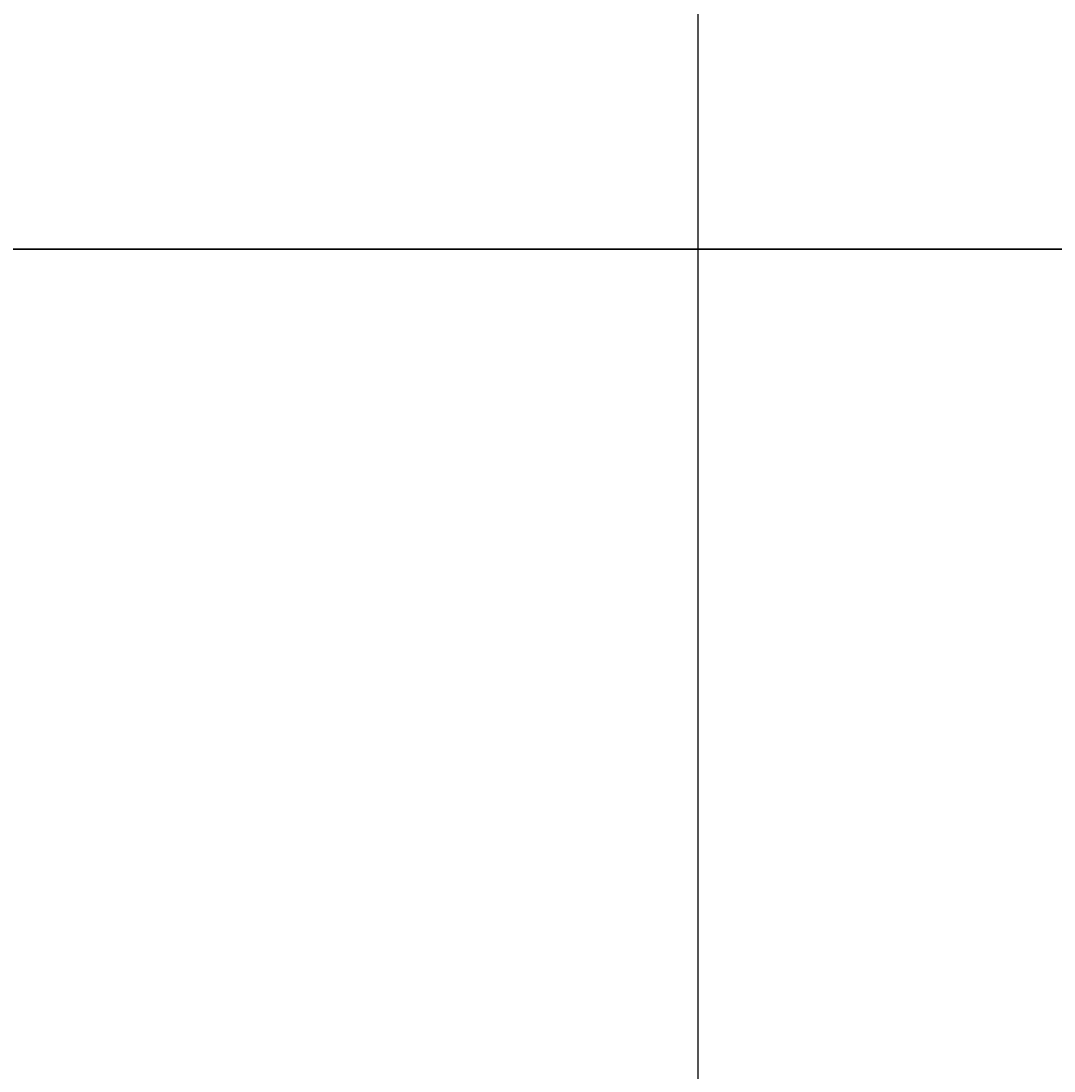
# Model space of a CAD drawing. Units: inches. Extents: x -6 to 289, y -8 to 323.
# Tile 82 of 107: x 173 to 196, y 229 to 252. Entities that reach past the tile are written whole.
import ezdxf

# ---------------------------------------------------------------- set-up
doc = ezdxf.new("R2010")
doc.units = ezdxf.units.IN
doc.header["$MEASUREMENT"] = 0
doc.layers.add('A-ANNO-DIMS', color=2, linetype='Continuous', lineweight=18)
doc.layers.add('A-ELEV', color=7, linetype='Continuous', lineweight=35)
doc.styles.get("Standard").update_dxf_attribs({"font": 'arial.ttf'})
doc.dimstyles.get("Standard").update_dxf_attribs({"dimtxt": 0.18, "dimasz": 0.18, "dimexe": 0.18, "dimexo": 0.0625, "dimgap": 0.09, "dimtad": 0, "dimtih": 1, "dimtoh": 1, "dimdec": 4, "dimzin": 0, "dimdsep": 46, "dimtxsty": 'Standard', "dimcen": 0.09, "dimadec": 0, "dimazin": 0, "dimtfac": 1, "dimtdec": 4, "dimtofl": 0, "dimtmove": 0, "dimatfit": 3, "dimfxl": 1, "dimtolj": 1, "dimtzin": 0, "dimarcsym": 0})

# ---------------------------------------------------------------- blocks, each defined once
blk = doc.blocks.new('*D12')
at = {"layer": 'A-ANNO-DIMS', "color": 0, "lineweight": -2, "transparency": 16777216}
for p, q in [((168.883, 226.717), (168.883, 322.969)), ((188.292, 226.951), (188.292, 322.969)), ((169.063, 322.789), (178.22, 322.789)), ((188.112, 322.789), (178.955, 322.789))]:
    blk.add_line(p, q, dxfattribs=at)
at = {"layer": 'A-ANNO-DIMS', "color": 0, "transparency": 16777216}
for points in [[(169.063, 322.819), (169.063, 322.759), (168.883, 322.789)], [(188.112, 322.819), (188.112, 322.759), (188.292, 322.789)]]:
    blk.add_solid(points, dxfattribs=at)
at = {"layer": 'Defpoints', "color": 0, "transparency": 16777216}
for p in [(188.292, 322.789), (188.292, 226.889), (168.883, 226.654)]:
    blk.add_point(p, dxfattribs=at)
at = {"layer": 'A-ANNO-DIMS', "color": 0, "transparency": 16777216, "insert": (178.588, 322.789), "char_height": 0.18, "attachment_point": 5}
blk.add_mtext('\\A1;19.41', dxfattribs=at)
blk = doc.blocks.new('*D13')
at = {"layer": 'A-ANNO-DIMS', "color": 0, "lineweight": -2, "transparency": 16777216}
for p, q in [((188.292, 226.951), (188.292, 322.969)), ((236.292, 226.951), (236.292, 322.969)), ((188.472, 322.789), (212.069, 322.789)), ((236.112, 322.789), (212.515, 322.789))]:
    blk.add_line(p, q, dxfattribs=at)
at = {"layer": 'A-ANNO-DIMS', "color": 0, "transparency": 16777216}
for points in [[(188.472, 322.819), (188.472, 322.759), (188.292, 322.789)], [(236.112, 322.819), (236.112, 322.759), (236.292, 322.789)]]:
    blk.add_solid(points, dxfattribs=at)
at = {"layer": 'Defpoints', "color": 0, "transparency": 16777216}
for p in [(236.292, 322.789), (188.292, 226.889), (236.292, 226.889)]:
    blk.add_point(p, dxfattribs=at)
at = {"layer": 'A-ANNO-DIMS', "color": 0, "transparency": 16777216, "insert": (212.292, 322.789), "char_height": 0.18, "attachment_point": 5}
blk.add_mtext('\\A1;48', dxfattribs=at)
blk = doc.blocks.new('*D26')
at = {"layer": 'A-ANNO-DIMS', "color": 0, "lineweight": -2, "transparency": 16777216}
for p, q in [((247.226, 247.289), (288.653, 247.289)), ((288.473, 247.109), (288.473, 237.153)), ((288.473, 226.834), (288.473, 236.789)), ((126.946, 226.654), (288.653, 226.654))]:
    blk.add_line(p, q, dxfattribs=at)
at = {"layer": 'A-ANNO-DIMS', "color": 0, "transparency": 16777216}
for points in [[(288.443, 247.109), (288.503, 247.109), (288.473, 247.289)], [(288.443, 226.834), (288.503, 226.834), (288.473, 226.654)]]:
    blk.add_solid(points, dxfattribs=at)
at = {"layer": 'Defpoints', "color": 0, "transparency": 16777216}
for p in [(247.164, 247.289), (288.473, 247.289), (126.883, 226.654)]:
    blk.add_point(p, dxfattribs=at)
at = {"layer": 'A-ANNO-DIMS', "color": 0, "transparency": 16777216, "insert": (288.473, 236.971), "char_height": 0.18, "attachment_point": 5}
blk.add_mtext('\\A1;20.635', dxfattribs=at)
blk = doc.blocks.new('*D27')
at = {"layer": 'A-ANNO-DIMS', "color": 0, "lineweight": -2, "transparency": 16777216}
for p, q in [((19.226, 307.289), (288.653, 307.289)), ((288.473, 307.109), (288.473, 277.471)), ((288.473, 247.469), (288.473, 277.107)), ((247.226, 247.289), (288.653, 247.289))]:
    blk.add_line(p, q, dxfattribs=at)
at = {"layer": 'A-ANNO-DIMS', "color": 0, "transparency": 16777216}
for points in [[(288.443, 307.109), (288.503, 307.109), (288.473, 307.289)], [(288.443, 247.469), (288.503, 247.469), (288.473, 247.289)]]:
    blk.add_solid(points, dxfattribs=at)
at = {"layer": 'Defpoints', "color": 0, "transparency": 16777216}
for p in [(19.164, 307.289), (288.473, 307.289), (247.164, 247.289)]:
    blk.add_point(p, dxfattribs=at)
at = {"layer": 'A-ANNO-DIMS', "color": 0, "transparency": 16777216, "insert": (288.473, 277.289), "char_height": 0.18, "attachment_point": 5}
blk.add_mtext('\\A1;60', dxfattribs=at)
blk = doc.blocks.new('*D79')
at = {"layer": 'A-ANNO-DIMS', "color": 0, "lineweight": -2, "transparency": 16777216}
for p, q in [((171.296, 118.033), (171.296, 322.969)), ((188.292, 116.842), (188.292, 322.969)), ((171.476, 322.789), (179.339, 322.789)), ((188.112, 322.789), (180.249, 322.789))]:
    blk.add_line(p, q, dxfattribs=at)
at = {"layer": 'A-ANNO-DIMS', "color": 0, "transparency": 16777216}
for points in [[(171.476, 322.819), (171.476, 322.759), (171.296, 322.789)], [(188.112, 322.819), (188.112, 322.759), (188.292, 322.789)]]:
    blk.add_solid(points, dxfattribs=at)
at = {"layer": 'Defpoints', "color": 0, "transparency": 16777216}
for p in [(188.292, 322.789), (171.296, 117.971), (188.292, 116.779)]:
    blk.add_point(p, dxfattribs=at)
at = {"layer": 'A-ANNO-DIMS', "color": 0, "transparency": 16777216, "insert": (179.794, 322.789), "char_height": 0.18, "attachment_point": 5}
blk.add_mtext('\\A1;16.996', dxfattribs=at)
blk = doc.blocks.new('*D80')
at = {"layer": 'A-ANNO-DIMS', "color": 0, "lineweight": -2, "transparency": 16777216}
for p, q in [((188.292, 116.842), (188.292, 322.969)), ((230.292, 116.842), (230.292, 322.969)), ((188.472, 322.789), (209.07, 322.789)), ((230.112, 322.789), (209.513, 322.789))]:
    blk.add_line(p, q, dxfattribs=at)
at = {"layer": 'A-ANNO-DIMS', "color": 0, "transparency": 16777216}
for points in [[(188.472, 322.819), (188.472, 322.759), (188.292, 322.789)], [(230.112, 322.819), (230.112, 322.759), (230.292, 322.789)]]:
    blk.add_solid(points, dxfattribs=at)
at = {"layer": 'Defpoints', "color": 0, "transparency": 16777216}
for p in [(230.292, 322.789), (188.292, 116.779), (230.292, 116.779)]:
    blk.add_point(p, dxfattribs=at)
at = {"layer": 'A-ANNO-DIMS', "color": 0, "transparency": 16777216, "insert": (209.292, 322.789), "char_height": 0.18, "attachment_point": 5}
blk.add_mtext('\\A1;42', dxfattribs=at)
blk = doc.blocks.new('*D96')
at = {"layer": 'A-ANNO-DIMS', "color": 0, "lineweight": -2, "transparency": 16777216}
for p, q in [((164.004, 159.411), (164.004, 322.969)), ((200.616, 159.411), (200.616, 322.969)), ((164.184, 322.789), (181.934, 322.789)), ((200.436, 322.789), (182.686, 322.789))]:
    blk.add_line(p, q, dxfattribs=at)
at = {"layer": 'A-ANNO-DIMS', "color": 0, "transparency": 16777216}
for points in [[(164.184, 322.819), (164.184, 322.759), (164.004, 322.789)], [(200.436, 322.819), (200.436, 322.759), (200.616, 322.789)]]:
    blk.add_solid(points, dxfattribs=at)
at = {"layer": 'Defpoints', "color": 0, "transparency": 16777216}
for p in [(200.616, 322.789), (164.004, 159.348), (200.616, 159.348)]:
    blk.add_point(p, dxfattribs=at)
at = {"layer": 'A-ANNO-DIMS', "color": 0, "transparency": 16777216, "insert": (182.31, 322.789), "char_height": 0.18, "attachment_point": 5}
blk.add_mtext('\\A1;36.61', dxfattribs=at)

msp = doc.modelspace()

# ---------------------------------------------------------------- linework, layer by layer
at = {"layer": 'A-ELEV'}
for p, q in [((247.1638, 247.2888), (115.1638, 247.2888)), ((115.1638, 247.2888), (247.1638, 247.2888))]:
    msp.add_line(p, q, dxfattribs=at)

# ---------------------------------------------------------------- dimensions: what is measured, and where the dimension line sits
at = {"layer": 'A-ANNO-DIMS'}
for base, p1, p2, override, picture, middle in [((200.6162, 322.7888), (164.0039, 159.3484), (200.6162, 159.3484), {"dimdec": 2, "dimlfac": 1, "dimrnd": 0, "dimzin": 0, "dimdsep": 46, "dimlunit": 2}, '*D96', (182.3101, 322.7888)), ((188.2918, 322.7888), (168.8835, 226.654), (188.2918, 226.8887), {"dimdec": 2, "dimlfac": 1, "dimrnd": 0, "dimzin": 0, "dimdsep": 46, "dimlunit": 2}, '*D12', (178.5876, 322.7888)), ((188.2918, 322.7888), (171.296, 117.9706), (188.2918, 116.7795), {"dimdec": 3, "dimlfac": 1, "dimrnd": 0, "dimzin": 0, "dimdsep": 46, "dimlunit": 2}, '*D79', (179.7939, 322.7888)), ((236.2918, 322.7888), (188.2918, 226.8887), (236.2918, 226.8887), {"dimdec": 0, "dimlfac": 1, "dimrnd": 0, "dimzin": 0, "dimdsep": 46, "dimlunit": 2}, '*D13', (212.2918, 322.7888)), ((230.2918, 322.7888), (188.2918, 116.7795), (230.2918, 116.7795), {"dimdec": 0, "dimlfac": 1, "dimrnd": 0, "dimzin": 0, "dimdsep": 46, "dimlunit": 2}, '*D80', (209.2918, 322.7888))]:
    dim = msp.add_linear_dim(base=base, p1=p1, p2=p2, dimstyle='Standard', override=override, dxfattribs=at)
    dim.commit()
    dim.dimension.update_dxf_attribs({"geometry": picture, "text_midpoint": middle})
for base, p1, p2, override, picture, middle in [((288.4733, 307.2888), (247.1638, 247.2888), (19.1638, 307.2888), {"dimdec": 0, "dimlfac": 1, "dimrnd": 0, "dimzin": 0, "dimdsep": 46, "dimlunit": 2}, '*D27', (288.4733, 277.2888)), ((288.4733, 247.2888), (126.8835, 226.654), (247.1638, 247.2888), {"dimdec": 3, "dimlfac": 1, "dimrnd": 0, "dimzin": 0, "dimdsep": 46, "dimlunit": 2}, '*D26', (288.4733, 236.9714))]:
    dim = msp.add_linear_dim(base=base, p1=p1, p2=p2, angle=90, dimstyle='Standard', override=override, dxfattribs=at)
    dim.commit()
    dim.dimension.update_dxf_attribs({"geometry": picture, "text_midpoint": middle})

doc.saveas('drawing.dxf')
